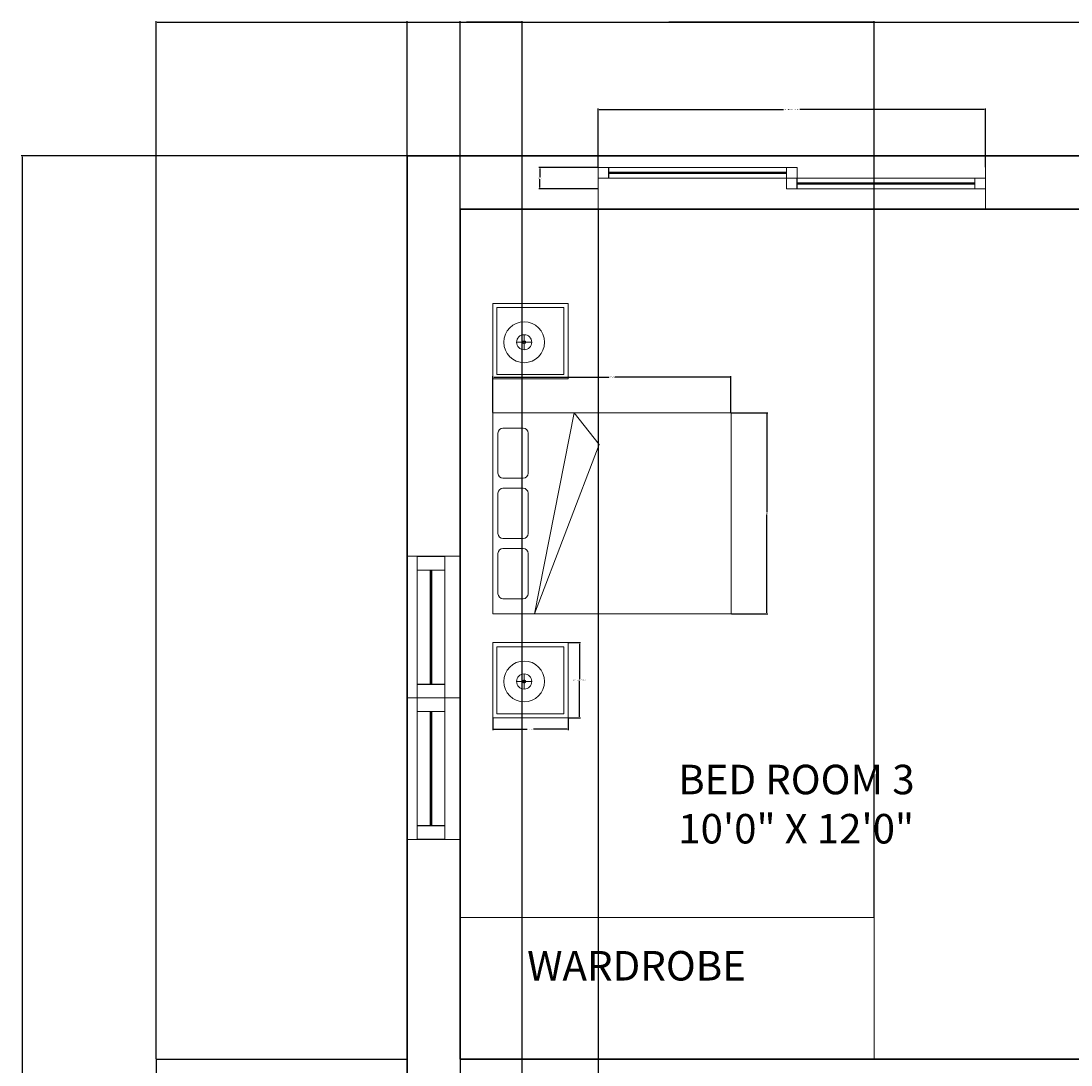
# Model space of a CAD drawing. Units: inches. Extents: x 1723 to 2209, y 1326 to 1810.
# Tile 3 of 6: x 1723 to 1901, y 1633 to 1810. Entities that reach past the tile are written whole.
import ezdxf

# ---------------------------------------------------------------- set-up
doc = ezdxf.new("R2010")
doc.units = ezdxf.units.IN
doc.layers.get('Defpoints').update_dxf_attribs({"color": 255})
for name, color, linetype, lineweight in [('A-ANNO-DIMS', 2, 'Continuous', 18), ('A-ANNO-TEXT', 7, 'Continuous', 18), ('A-AREA-IDEN', 7, 'Continuous', 18), ('A-FLOR', 7, 'Continuous', 25), ('A-FLOR-CASE', 9, 'Continuous', 18), ('A-FURN', 8, 'Continuous', 13), ('A-GLAZ', 4, 'Continuous', 18), ('A-WALL', 7, 'Continuous', 35), ('Sliding Door', 3, 'Continuous', 18)]:
    doc.layers.add(name, color=color, linetype=linetype, lineweight=lineweight)
doc.styles.get("Standard").update_dxf_attribs({"font": 'arial.ttf'})
doc.dimstyles.get("Standard").update_dxf_attribs({"dimtxt": 0.18, "dimasz": 0.18, "dimexe": 0.18, "dimexo": 0.0625, "dimgap": 0.09, "dimtad": 0, "dimtih": 1, "dimtoh": 1, "dimdec": 4, "dimzin": 0, "dimdsep": 46, "dimtxsty": 'Standard', "dimcen": 0.09, "dimadec": 0, "dimazin": 0, "dimtfac": 1, "dimtdec": 4, "dimtofl": 0, "dimtmove": 0, "dimatfit": 3, "dimfxl": 1, "dimtolj": 1, "dimtzin": 0, "dimarcsym": 0})

# ---------------------------------------------------------------- blocks, each defined once
blk = doc.blocks.new('A$C793B20D3')
for p, q in [((0.625, -0.395), (0.625, 1.975)), ((2.625, 1.975), (0.625, 1.975)), ((0.825, 1.925), (1.225, 1.925)), ((1.425, 1.925), (1.825, 1.925)), ((2.025, 1.925), (2.425, 1.925)), ((2.625, -0.395), (2.625, 1.975)), ((0.775, 1.675), (0.775, 1.875)), ((1.275, 1.675), (1.275, 1.875)), ((1.375, 1.675), (1.375, 1.875)), ((1.875, 1.675), (1.875, 1.875)), ((1.975, 1.675), (1.975, 1.875)), ((2.475, 1.675), (2.475, 1.875)), ((0.825, 1.625), (1.225, 1.625)), ((1.425, 1.625), (1.825, 1.625)), ((2.025, 1.625), (2.425, 1.625)), ((0.626, 1.56), (2.311, 0.917)), ((0.626, 1.56), (2.625, 1.165)), ((2.311, 0.917), (2.625, 1.165)), ((2.625, -0.395), (0.625, -0.395))]:
    blk.add_line(p, q)
for centre, start, end in [((0.825, 1.875), 90, 180), ((1.225, 1.875), 0, 90), ((1.425, 1.875), 90, 180), ((1.825, 1.875), 0, 90), ((2.025, 1.875), 90, 180), ((2.425, 1.875), 0, 90), ((0.825, 1.675), 180, 270), ((1.225, 1.675), 270, 0), ((1.425, 1.675), 180, 270), ((1.825, 1.675), 270, 0), ((2.025, 1.675), 180, 270), ((2.425, 1.675), 270, 0)]:
    blk.add_arc(centre, 0.05, start, end)
blk = doc.blocks.new('A$C7a76cbd6')
at = {"layer": 'Sliding Door'}
for p, q in [((540.4, 283.7, 0), (478.3, 283.7, 0)), ((478.3, 283.7, 0), (540.4, 283.7, 0)), ((540.4, 221.5, 0), (540.4, 283.7, 0)), ((540.4, 283.7, 0), (1585.3, 283.7, 0)), ((540.4, 283.7, 0), (540.4, 221.5, 0)), ((1585.3, 256.6, 0), (540.4, 256.6, 0)), ((540.4, 256.6, 0), (540.4, 248.7, 0)), ((540.4, 252.6, 0), (1584.3, 252.6, 0)), ((540.4, 248.7, 0), (1585.3, 248.7, 0)), ((1584.3, 283.7, 0), (1647.4, 283.7, 0)), ((1584.3, 283.7, 0), (1584.3, 221.5, 0)), ((1647.4, 283.7, 0), (1585.3, 283.7, 0)), ((1585.3, 283.7, 0), (1585.3, 221.5, 0)), ((1585.3, 248.7, 0), (1585.3, 256.6, 0)), ((1647.4, 221.5, 0), (1647.4, 283.7, 0)), ((1647.4, 283.7, 0), (1647.4, 221.5, 0)), ((478.3, 221.5, 0), (540.4, 221.5, 0)), ((478.3, 221.5, 0), (540.4, 221.5, 0)), ((1584.3, 221.5, 0), (540.4, 221.5, 0)), ((1646.4, 221.5, 0), (1584.3, 221.5, 0)), ((1584.3, 221.5, 0), (1584.3, 159.4, 0)), ((1584.3, 221.5, 0), (1647.4, 221.5, 0)), ((1584.3, 221.5, 0), (1647.4, 221.5, 0)), ((1584.3, 221.5, 0), (1584.3, 159.4, 0)), ((1585.3, 221.5, 0), (1647.4, 221.5, 0)), ((1646.4, 159.4, 0), (1646.4, 221.5, 0)), ((1647.4, 221.5, 0), (2691.3, 221.5, 0)), ((1647.4, 221.5, 0), (1647.4, 159.4, 0)), ((2691.3, 194.4, 0), (1647.4, 194.4, 0)), ((1647.4, 194.4, 0), (1647.4, 186.5, 0)), ((1647.4, 190.5, 0), (2690.3, 190.5, 0)), ((1647.4, 186.5, 0), (2691.3, 186.5, 0)), ((2690.3, 221.5, 0), (2753.4, 221.5, 0)), ((2690.3, 221.5, 0), (2690.3, 159.4, 0)), ((2753.4, 221.5, 0), (2691.3, 221.5, 0)), ((2691.3, 221.5, 0), (2691.3, 159.4, 0)), ((2691.3, 186.5, 0), (2691.3, 194.4, 0)), ((1584.3, 159.4, 0), (1646.4, 159.4, 0)), ((1584.3, 159.4, 0), (1647.4, 159.4, 0)), ((2691.3, 159.4, 0), (1646.4, 159.4, 0)), ((2690.3, 159.4, 0), (2753.4, 159.4, 0)), ((2691.3, 159.4, 0), (2753.4, 159.4, 0))]:
    blk.add_line(p, q, dxfattribs=at)
blk = doc.blocks.new('SW')
blk.add_line((2331.37, 1559.31), (2331.37, 1550.31))
at = {"layer": 'Sliding Door'}
for p, q in [((2285.07, 1559.31), (2285.07, 1550.31)), ((2285.07, 1559.31), (2285.07, 1550.31)), ((2285.07, 1559.31), (2289.58, 1559.31)), ((2289.51, 1550.31), (2289.51, 1559.31)), ((2331.37, 1559.31), (2289.51, 1559.31)), ((2289.58, 1559.31), (2289.58, 1550.31)), ((2326.86, 1559.31), (2326.86, 1550.31)), ((2326.86, 1559.31), (2331.37, 1559.31)), ((2326.93, 1559.31), (2326.93, 1550.31)), ((2326.86, 1555.09), (2289.58, 1555.09)), ((2289.58, 1554.81), (2326.86, 1554.81)), ((2289.58, 1554.53), (2326.86, 1554.53)), ((2285.07, 1550.31), (2289.51, 1550.31)), ((2285.07, 1550.31), (2289.58, 1550.31)), ((2331.37, 1550.31), (2289.51, 1550.31)), ((2289.58, 1552.81), (2289.58, 1552.25)), ((2326.86, 1550.31), (2331.37, 1550.31)), ((2326.93, 1552.25), (2326.93, 1552.81)), ((2326.93, 1550.31), (2331.37, 1550.31))]:
    blk.add_line(p, q, dxfattribs=at)
blk = doc.blocks.new('TABLE-END-SMALL')
for p, q in [((5.32, 4.88), (5.32, 7.45)), ((6.6, 6.17), (4.03, 6.17))]:
    blk.add_line(p, q)
for points in [[(0, 0), (12.75, 0), (12.75, 12.75), (0, 12.75)], [(0.71, 0.71), (12.04, 0.71), (12.04, 12.04), (0.71, 12.04)]]:
    blk.add_lwpolyline(points, close=True)
for radius in [3.46, 1.28, 0.266]:
    blk.add_circle((5.32, 6.17), radius)
blk = doc.blocks.new('*D57')
at = {"layer": 'A-ANNO-DIMS', "color": 0, "lineweight": -2, "transparency": 16777216}
for p, q in [((1815.43, 1704.24), (1817.46, 1704.24)), ((1817.28, 1704.06), (1817.28, 1698.05)), ((1817.28, 1691.67), (1817.28, 1697.69)), ((1815.43, 1691.49), (1817.46, 1691.49))]:
    blk.add_line(p, q, dxfattribs=at)
at = {"layer": 'A-ANNO-DIMS', "color": 0, "transparency": 16777216}
for points in [[(1817.25, 1704.06), (1817.31, 1704.06), (1817.28, 1704.24)], [(1817.25, 1691.67), (1817.31, 1691.67), (1817.28, 1691.49)]]:
    blk.add_solid(points, dxfattribs=at)
at = {"layer": 'Defpoints', "color": 0, "transparency": 16777216}
for p in [(1815.37, 1704.24), (1817.28, 1704.24), (1815.37, 1691.49)]:
    blk.add_point(p, dxfattribs=at)
at = {"layer": 'A-ANNO-DIMS', "color": 0, "transparency": 16777216, "insert": (1817.28, 1697.87), "char_height": 0.18, "attachment_point": 5}
blk.add_mtext('\\A1;END TABLE 13 TYP.', dxfattribs=at)
blk = doc.blocks.new('*D58')
at = {"layer": 'A-ANNO-DIMS', "color": 0, "lineweight": -2, "transparency": 16777216}
for p, q in [((1802.61, 1691.43), (1802.61, 1689.4)), ((1815.37, 1691.43), (1815.37, 1689.4)), ((1802.79, 1689.58), (1808.47, 1689.58)), ((1815.19, 1689.58), (1809.51, 1689.58))]:
    blk.add_line(p, q, dxfattribs=at)
at = {"layer": 'A-ANNO-DIMS', "color": 0, "transparency": 16777216}
for points in [[(1802.79, 1689.61), (1802.79, 1689.55), (1802.61, 1689.58)], [(1815.19, 1689.61), (1815.19, 1689.55), (1815.37, 1689.58)]]:
    blk.add_solid(points, dxfattribs=at)
at = {"layer": 'Defpoints', "color": 0, "transparency": 16777216}
for p in [(1802.61, 1691.49), (1815.37, 1691.49), (1815.37, 1689.58)]:
    blk.add_point(p, dxfattribs=at)
at = {"layer": 'A-ANNO-DIMS', "color": 0, "transparency": 16777216, "insert": (1808.99, 1689.58), "char_height": 0.18, "attachment_point": 5}
blk.add_mtext('\\A1;13 TYP.', dxfattribs=at)
blk = doc.blocks.new('*D65')
at = {"layer": 'A-ANNO-DIMS', "color": 0, "lineweight": -2, "transparency": 16777216}
for p, q in [((1820.45, 1784.78), (1820.45, 1794.73)), ((1820.63, 1794.55), (1851.85, 1794.55)), ((1885.85, 1794.55), (1854.64, 1794.55)), ((1886.03, 1784.78), (1886.03, 1794.73))]:
    blk.add_line(p, q, dxfattribs=at)
at = {"layer": 'A-ANNO-DIMS', "color": 0, "transparency": 16777216}
for points in [[(1820.63, 1794.58), (1820.63, 1794.52), (1820.45, 1794.55)], [(1885.85, 1794.58), (1885.85, 1794.52), (1886.03, 1794.55)]]:
    blk.add_solid(points, dxfattribs=at)
at = {"layer": 'Defpoints', "color": 0, "transparency": 16777216}
for p in [(1820.45, 1794.55), (1820.45, 1784.71), (1886.03, 1784.71)]:
    blk.add_point(p, dxfattribs=at)
at = {"layer": 'A-ANNO-DIMS', "color": 0, "transparency": 16777216, "insert": (1853.24, 1794.55), "char_height": 0.18, "attachment_point": 5}
blk.add_mtext('\\A1;SLIDING UNIT 66 TYP.', dxfattribs=at)
blk = doc.blocks.new('*D66')
at = {"layer": 'A-ANNO-DIMS', "color": 0, "lineweight": -2, "transparency": 16777216}
for p, q in [((1820.39, 1784.71), (1810.43, 1784.71)), ((1810.61, 1784.53), (1810.61, 1783.1)), ((1810.61, 1781.31), (1810.61, 1782.74)), ((1820.39, 1781.13), (1810.43, 1781.13))]:
    blk.add_line(p, q, dxfattribs=at)
at = {"layer": 'A-ANNO-DIMS', "color": 0, "transparency": 16777216}
for points in [[(1810.58, 1784.53), (1810.64, 1784.53), (1810.61, 1784.71)], [(1810.58, 1781.31), (1810.64, 1781.31), (1810.61, 1781.13)]]:
    blk.add_solid(points, dxfattribs=at)
at = {"layer": 'Defpoints', "color": 0, "transparency": 16777216}
for p in [(1820.45, 1784.71), (1810.61, 1781.13), (1820.45, 1781.13)]:
    blk.add_point(p, dxfattribs=at)
at = {"layer": 'A-ANNO-DIMS', "color": 0, "transparency": 16777216, "insert": (1810.61, 1782.92), "char_height": 0.18, "attachment_point": 5}
blk.add_mtext('\\A1;4 TYP.', dxfattribs=at)
blk = doc.blocks.new('*D69')
at = {"layer": 'A-ANNO-DIMS', "color": 0, "lineweight": -2, "transparency": 16777216}
for p, q in [((1802.64, 1743.21), (1802.64, 1749.37)), ((1802.82, 1749.19), (1822.29, 1749.19)), ((1842.77, 1749.19), (1823.31, 1749.19)), ((1842.95, 1743.21), (1842.95, 1749.37))]:
    blk.add_line(p, q, dxfattribs=at)
at = {"layer": 'A-ANNO-DIMS', "color": 0, "transparency": 16777216}
for points in [[(1802.82, 1749.22), (1802.82, 1749.16), (1802.64, 1749.19)], [(1842.77, 1749.22), (1842.77, 1749.16), (1842.95, 1749.19)]]:
    blk.add_solid(points, dxfattribs=at)
at = {"layer": 'Defpoints', "color": 0, "transparency": 16777216}
for p in [(1802.64, 1749.19), (1802.64, 1743.15), (1842.95, 1743.15)]:
    blk.add_point(p, dxfattribs=at)
at = {"layer": 'A-ANNO-DIMS', "color": 0, "transparency": 16777216, "insert": (1822.8, 1749.19), "char_height": 0.18, "attachment_point": 5}
blk.add_mtext('\\A1;BED 40', dxfattribs=at)
blk = doc.blocks.new('*D70')
at = {"layer": 'A-ANNO-DIMS', "color": 0, "lineweight": -2, "transparency": 16777216}
for p, q in [((1843.02, 1743.15), (1849.18, 1743.15)), ((1849, 1742.97), (1849, 1726.32)), ((1849, 1709.3), (1849, 1725.95)), ((1843.02, 1709.12), (1849.18, 1709.12))]:
    blk.add_line(p, q, dxfattribs=at)
at = {"layer": 'A-ANNO-DIMS', "color": 0, "transparency": 16777216}
for points in [[(1848.97, 1742.97), (1849.03, 1742.97), (1849, 1743.15)], [(1848.97, 1709.3), (1849.03, 1709.3), (1849, 1709.12)]]:
    blk.add_solid(points, dxfattribs=at)
at = {"layer": 'Defpoints', "color": 0, "transparency": 16777216}
for p in [(1842.95, 1743.15), (1849, 1743.15), (1842.95, 1709.12)]:
    blk.add_point(p, dxfattribs=at)
at = {"layer": 'A-ANNO-DIMS', "color": 0, "transparency": 16777216, "insert": (1849, 1726.14), "char_height": 0.18, "attachment_point": 5}
blk.add_mtext('\\A1;34', dxfattribs=at)
blk = doc.blocks.new('*D93')
at = {"layer": 'A-ANNO-DIMS', "color": 0, "lineweight": -2, "transparency": 16777216}
for p, q in [((1745.6, 1633.75), (1745.6, 1809.54)), ((1745.78, 1809.36), (1965.31, 1809.36)), ((2185.42, 1809.36), (1965.9, 1809.36)), ((2185.6, 1786.75), (2185.6, 1809.54))]:
    blk.add_line(p, q, dxfattribs=at)
at = {"layer": 'A-ANNO-DIMS', "color": 0, "transparency": 16777216}
for points in [[(1745.78, 1809.39), (1745.78, 1809.33), (1745.6, 1809.36)], [(2185.42, 1809.39), (2185.42, 1809.33), (2185.6, 1809.36)]]:
    blk.add_solid(points, dxfattribs=at)
at = {"layer": 'Defpoints', "color": 0, "transparency": 16777216}
for p in [(2185.6, 1809.36), (2185.6, 1786.69), (1745.6, 1633.69)]:
    blk.add_point(p, dxfattribs=at)
at = {"layer": 'A-ANNO-DIMS', "color": 0, "transparency": 16777216, "insert": (1965.6, 1809.36), "char_height": 0.18, "attachment_point": 5}
blk.add_mtext('\\A1;440', dxfattribs=at)
blk = doc.blocks.new('*D94')
at = {"layer": 'A-ANNO-DIMS', "color": 0, "lineweight": -2, "transparency": 16777216}
for p, q in [((1788.04, 1786.69), (1722.75, 1786.69)), ((1722.93, 1786.51), (1722.93, 1567.87)), ((1722.93, 1348.87), (1722.93, 1567.51)), ((1788.04, 1348.69), (1722.75, 1348.69))]:
    blk.add_line(p, q, dxfattribs=at)
at = {"layer": 'A-ANNO-DIMS', "color": 0, "transparency": 16777216}
for points in [[(1722.9, 1786.51), (1722.96, 1786.51), (1722.93, 1786.69)], [(1722.9, 1348.87), (1722.96, 1348.87), (1722.93, 1348.69)]]:
    blk.add_solid(points, dxfattribs=at)
at = {"layer": 'Defpoints', "color": 0, "transparency": 16777216}
for p in [(1722.93, 1786.69), (1788.1, 1786.69), (1788.1, 1348.69)]:
    blk.add_point(p, dxfattribs=at)
at = {"layer": 'A-ANNO-DIMS', "color": 0, "transparency": 16777216, "insert": (1722.93, 1567.69), "char_height": 0.18, "attachment_point": 5}
blk.add_mtext('\\A1;438', dxfattribs=at)
blk = doc.blocks.new('*D110')
at = {"layer": 'A-ANNO-DIMS', "color": 0, "lineweight": -2, "transparency": 16777216}
for p, q in [((1788.1, 1506.25), (1788.1, 1809.54)), ((1788.28, 1809.36), (1797.54, 1809.36)), ((1807.42, 1809.36), (1798.17, 1809.36)), ((1807.6, 1506.25), (1807.6, 1809.54))]:
    blk.add_line(p, q, dxfattribs=at)
at = {"layer": 'A-ANNO-DIMS', "color": 0, "transparency": 16777216}
for points in [[(1788.28, 1809.39), (1788.28, 1809.33), (1788.1, 1809.36)], [(1807.42, 1809.39), (1807.42, 1809.33), (1807.6, 1809.36)]]:
    blk.add_solid(points, dxfattribs=at)
at = {"layer": 'Defpoints', "color": 0, "transparency": 16777216}
for p in [(1807.6, 1809.36), (1788.1, 1506.19), (1807.6, 1506.19)]:
    blk.add_point(p, dxfattribs=at)
at = {"layer": 'A-ANNO-DIMS', "color": 0, "transparency": 16777216, "insert": (1797.85, 1809.36), "char_height": 0.18, "attachment_point": 5}
blk.add_mtext('\\A1;19.5', dxfattribs=at)
blk = doc.blocks.new('*D112')
at = {"layer": 'A-ANNO-DIMS', "color": 0, "lineweight": -2, "transparency": 16777216}
for p, q in [((1797.1, 1657.75), (1797.1, 1809.54)), ((1797.28, 1809.36), (1831.85, 1809.36)), ((1867.02, 1809.36), (1832.46, 1809.36)), ((1867.2, 1657.75), (1867.2, 1809.54))]:
    blk.add_line(p, q, dxfattribs=at)
at = {"layer": 'A-ANNO-DIMS', "color": 0, "transparency": 16777216}
for points in [[(1797.28, 1809.39), (1797.28, 1809.33), (1797.1, 1809.36)], [(1867.02, 1809.39), (1867.02, 1809.33), (1867.2, 1809.36)]]:
    blk.add_solid(points, dxfattribs=at)
at = {"layer": 'Defpoints', "color": 0, "transparency": 16777216}
for p in [(1867.2, 1809.36), (1797.1, 1657.69), (1867.2, 1657.69)]:
    blk.add_point(p, dxfattribs=at)
at = {"layer": 'A-ANNO-DIMS', "color": 0, "transparency": 16777216, "insert": (1832.15, 1809.36), "char_height": 0.18, "attachment_point": 5}
blk.add_mtext('\\A1;70.1', dxfattribs=at)
blk = doc.blocks.new('*D114')
at = {"layer": 'A-ANNO-DIMS', "color": 0, "lineweight": -2, "transparency": 16777216}
for p, q in [((1797.1, 1777.63), (1797.1, 1325.84)), ((1820.45, 1777.63), (1820.45, 1325.84)), ((1797.28, 1326.02), (1808.38, 1326.02)), ((1820.27, 1326.02), (1809.17, 1326.02))]:
    blk.add_line(p, q, dxfattribs=at)
at = {"layer": 'A-ANNO-DIMS', "color": 0, "transparency": 16777216}
for points in [[(1797.28, 1326.05), (1797.28, 1325.99), (1797.1, 1326.02)], [(1820.27, 1326.05), (1820.27, 1325.99), (1820.45, 1326.02)]]:
    blk.add_solid(points, dxfattribs=at)
at = {"layer": 'Defpoints', "color": 0, "transparency": 16777216}
for p in [(1797.1, 1777.69), (1820.45, 1777.69), (1820.45, 1326.02)]:
    blk.add_point(p, dxfattribs=at)
at = {"layer": 'A-ANNO-DIMS', "color": 0, "transparency": 16777216, "insert": (1808.78, 1326.02), "char_height": 0.18, "attachment_point": 5}
blk.add_mtext('\\A1;23.35', dxfattribs=at)

msp = doc.modelspace()

# ---------------------------------------------------------------- linework, layer by layer
at = {"layer": 'A-FLOR'}
msp.add_line((1745.6032, 1633.6915), (1745.6032, 1487.6915), dxfattribs=at)
msp.add_lwpolyline([(1745.6032, 1633.6915), (1788.1032, 1633.6915)], dxfattribs=at)
at = {"layer": 'A-FLOR-CASE'}
for p, q in [((1797.1032, 1657.6915), (1867.202, 1657.6915)), ((1867.202, 1657.6915), (1867.202, 1633.6915))]:
    msp.add_line(p, q, dxfattribs=at)
at = {"layer": 'A-GLAZ'}
for p, q in [((1820.4509, 1786.6915), (1820.4509, 1777.6915)), ((1886.0318, 1786.6915), (1886.0318, 1777.6915))]:
    msp.add_line(p, q, dxfattribs=at)
for points in [[(1788.1032, 1718.8784), (1788.1032, 1694.8784), (1797.1032, 1694.8784), (1797.1032, 1718.8784)], [(1788.1032, 1670.8784), (1788.1032, 1694.8784), (1797.1032, 1694.8784), (1797.1032, 1670.8784)]]:
    msp.add_lwpolyline(points, close=True, dxfattribs=at)
at = {"layer": 'A-WALL'}
for p, q in [((1797.1032, 1777.6915), (1917.1032, 1777.6915)), ((1797.1032, 1777.6915), (1797.1032, 1633.6915)), ((1797.1032, 1633.6915), (1954.4027, 1633.6915))]:
    msp.add_line(p, q, dxfattribs=at)
msp.add_lwpolyline([(1788.1032, 1629.1915), (1788.1032, 1786.6915), (2185.6032, 1786.6915), (2185.6032, 1612.485)], dxfattribs=at)

# ---------------------------------------------------------------- block references
at = {"layer": 'A-FURN'}
for p in [(1802.6136, 1748.9535), (1802.6136, 1691.492)]:
    msp.add_blockref('TABLE-END-SMALL', p, dxfattribs=at)
at = {"layer": 'A-FURN', "xscale": 17.01157910559595, "yscale": 17.01157910559595, "zscale": 17.01157910559595, "rotation": 90}
msp.add_blockref('A$C793B20D3', (1836.2419, 1698.4923), dxfattribs=at)
at = {"layer": 'A-GLAZ'}
for name, p, xscale, yscale, zscale, rotation in [('A$C7a76cbd6', (1899.8174, 1789.309), 0.0288245099661422, 0.0288245099661422, 0.0288245099661422, 180), ('SW', (2596.7067, 2901.2814), -0.5174661543078929, 0.5174661543078929, 0.5174661543078929, 90), ('SW', (2596.7067, 488.4754), 0.5174661543078929, 0.5174661543078929, 0.5174661543078929, 90)]:
    msp.add_blockref(name, p, dxfattribs=dict(at, xscale=xscale, yscale=yscale, zscale=zscale, rotation=rotation))

# ---------------------------------------------------------------- texts
at = {"layer": 'A-ANNO-TEXT', "insert": (1808.4363, 1652.0029), "char_height": 5, "attachment_point": 1}
msp.add_mtext_dynamic_manual_height_columns('WARDROBE', width=43.999866, gutter_width=12.5, heights=[0], dxfattribs=at)
at = {"layer": 'A-AREA-IDEN', "insert": (1834.0243, 1683.551), "char_height": 5, "attachment_point": 1}
msp.add_mtext_dynamic_manual_height_columns('BED ROOM 3\\P10\'0" X 12\'0"', width=63.019392, gutter_width=12.5, heights=[0], dxfattribs=at)

# ---------------------------------------------------------------- dimensions: what is measured, and where the dimension line sits
at = {"layer": 'A-ANNO-DIMS'}
for base, p1, p2, override, picture, middle in [((2185.6032, 1809.3615), (1745.6032, 1633.6915), (2185.6032, 1786.6915), {"dimdec": 0, "dimlfac": 1, "dimrnd": 0, "dimzin": 0, "dimdsep": 46, "dimlunit": 2}, '*D93', (1965.6032, 1809.3615)), ((1807.6032, 1809.3615), (1788.1032, 1506.1915), (1807.6032, 1506.1915), {"dimdec": 1, "dimlfac": 1, "dimrnd": 0, "dimzin": 0, "dimdsep": 46, "dimlunit": 2}, '*D110', (1797.8532, 1809.3615)), ((1867.202, 1809.3615), (1797.1032, 1657.6915), (1867.202, 1657.6915), {"dimdec": 1, "dimlfac": 1, "dimrnd": 0, "dimzin": 0, "dimdsep": 46, "dimlunit": 2}, '*D112', (1832.1526, 1809.3615)), ((1820.4509, 1326.0215), (1797.1032, 1777.6915), (1820.4509, 1777.6915), {"dimdec": 2, "dimlfac": 1, "dimrnd": 0, "dimzin": 0, "dimdsep": 46, "dimlunit": 2}, '*D114', (1808.777, 1326.0215))]:
    dim = msp.add_linear_dim(base=base, p1=p1, p2=p2, dimstyle='Standard', override=override, dxfattribs=at)
    dim.commit()
    dim.dimension.update_dxf_attribs({"geometry": picture, "text_midpoint": middle})
for base, p1, p2, angle, text, picture, middle in [((1820.4509, 1794.5518), (1886.0318, 1784.7147), (1820.4509, 1784.7147), 180, 'SLIDING UNIT <> TYP.', '*D65', (1853.2414, 1794.5518)), ((1810.6138, 1781.1311), (1820.4509, 1784.7147), (1820.4509, 1781.1311), 270, '<> TYP.', '*D66', (1810.6138, 1782.9229)), ((1802.644, 1749.1942), (1842.9536, 1743.1478), (1802.644, 1743.1478), 180, 'BED <>', '*D69', (1822.7988, 1749.1942)), ((1817.2787, 1704.2443), (1815.3659, 1691.492), (1815.3659, 1704.2443), 90, 'END TABLE <> TYP.', '*D57', (1817.2787, 1697.8681))]:
    dim = msp.add_linear_dim(base=base, p1=p1, p2=p2, angle=angle, text=text, dimstyle='Standard', override={"dimdec": 0, "dimlfac": 1, "dimrnd": 0, "dimzin": 0, "dimdsep": 46, "dimlunit": 2}, dxfattribs=at)
    dim.commit()
    dim.dimension.update_dxf_attribs({"geometry": picture, "text_midpoint": middle})
for base, p1, p2, picture, middle in [((1722.9332, 1786.6915), (1788.1032, 1348.6915), (1788.1032, 1786.6915), '*D94', (1722.9332, 1567.6915)), ((1849, 1743.1478), (1842.9536, 1709.1246), (1842.9536, 1743.1478), '*D70', (1849, 1726.1362))]:
    dim = msp.add_linear_dim(base=base, p1=p1, p2=p2, angle=90, dimstyle='Standard', override={"dimdec": 0, "dimlfac": 1, "dimrnd": 0, "dimzin": 0, "dimdsep": 46, "dimlunit": 2}, dxfattribs=at)
    dim.commit()
    dim.dimension.update_dxf_attribs({"geometry": picture, "text_midpoint": middle})
dim = msp.add_linear_dim(base=(1815.3659, 1689.5791), p1=(1802.6136, 1691.492), p2=(1815.3659, 1691.492), text='<> TYP.', dimstyle='Standard', override={"dimdec": 0, "dimlfac": 1, "dimrnd": 0, "dimzin": 0, "dimdsep": 46, "dimlunit": 2}, dxfattribs=at)
dim.commit()
dim.dimension.update_dxf_attribs({"geometry": '*D58', "text_midpoint": (1808.9897, 1689.5791)})

doc.saveas('drawing.dxf')
